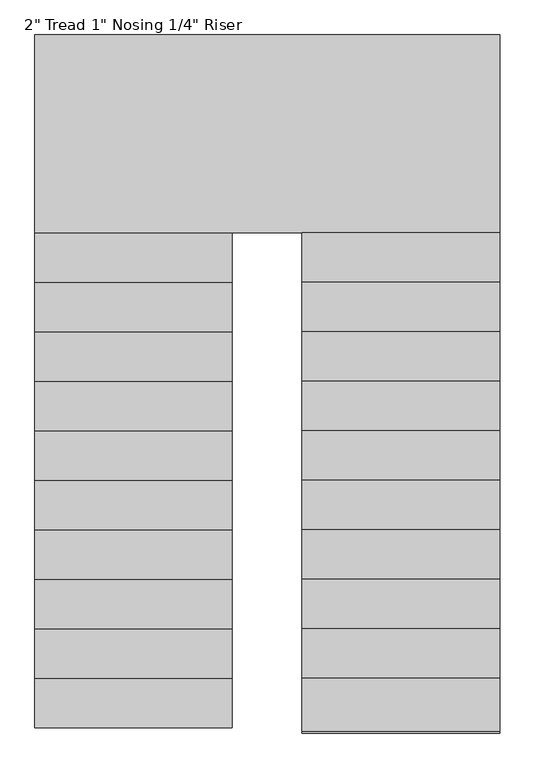
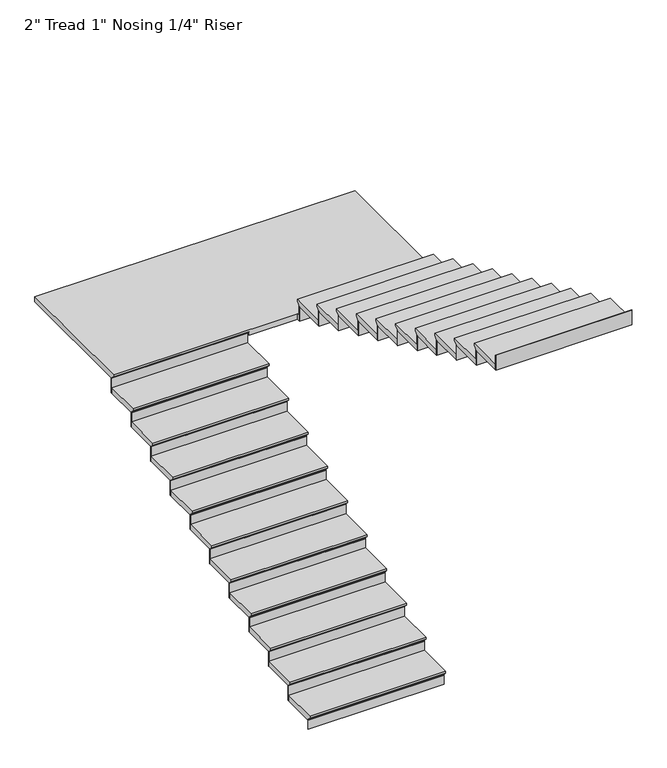
"""IFC4 building model written with IfcOpenShell, lengths in millimetres: stair flight geometry."""

from ifc_helpers import new_model, si_unit, origin, place, context, project, spatial, faceted_brep, source, transform, mapped, element, save


def stair_flight_f8c5991c(model_context):
    return source(origin(), model_context, "Body", "Brep", [
        faceted_brep([(-629.5987998, 3364.6067329, 3319.8954545), (-629.5987998, 3364.6067329, 3338.9454545), (-1845.5417538, 3364.6067329, 3338.9454545), (-1845.5417538, 3364.6067329, 3319.8954545), (-629.5987998, 3390.0067329, 3294.4954545), (-1845.5417538, 3390.0067329, 3294.4954545), (-629.5987998, 3694.8067329, 3338.9454545), (-1845.5417538, 3694.8067329, 3338.9454545), (-1845.5417538, 3390.0067329, 3288.1454545), (-1845.5417538, 3694.8067329, 3288.1454545), (-629.5987998, 3694.8067329, 3288.1454545), (-629.5987998, 3390.0067329, 3288.1454545)], [[[0, 1, 2, 3]], [[4, 0, 3, 5]], [[2, 1, 6, 7]], [[8, 9, 10, 11]], [[2, 7, 9, 8, 5, 3]], [[8, 11, 4, 5]], [[6, 1, 0, 4, 11, 10]], [[7, 6, 10, 9]]]),
        faceted_brep([(-629.5987998, 3390.0067329, 3288.1454545), (-629.5987998, 3390.0067329, 3200.4), (-629.5987998, 3396.3567329, 3200.4), (-629.5987998, 3396.3567329, 3288.1454545), (-1845.5417538, 3390.0067329, 3288.1454545), (-1845.5417538, 3396.3567329, 3288.1454545), (-1845.5417538, 3396.3567329, 3200.4), (-1845.5417538, 3390.0067329, 3200.4)], [[[0, 1, 2, 3]], [[4, 5, 6, 7]], [[1, 0, 4, 7]], [[2, 1, 7, 6]], [[3, 2, 6, 5]], [[0, 3, 5, 4]]]),
        faceted_brep([(-629.5987998, 3694.8067329, 3426.6909091), (-629.5987998, 3694.8067329, 3288.1454545), (-629.5987998, 3701.1567329, 3288.1454545), (-629.5987998, 3701.1567329, 3426.6909091), (-1845.5417538, 3694.8067329, 3426.6909091), (-1845.5417538, 3701.1567329, 3426.6909091), (-1845.5417538, 3701.1567329, 3288.1454545), (-1845.5417538, 3694.8067329, 3288.1454545)], [[[0, 1, 2, 3]], [[4, 5, 6, 7]], [[1, 0, 4, 7]], [[2, 1, 7, 6]], [[3, 2, 6, 5]], [[0, 3, 5, 4]]]),
        faceted_brep([(-1845.5417538, 3669.4067329, 3477.4909091), (-629.5987998, 3669.4067329, 3477.4909091), (-629.5987998, 3999.6067329, 3477.4909091), (-1845.5417538, 3999.6067329, 3477.4909091), (-1845.5417538, 3694.8067329, 3426.6909091), (-1845.5417538, 3999.6067329, 3426.6909091), (-629.5987998, 3999.6067329, 3426.6909091), (-629.5987998, 3694.8067329, 3426.6909091), (-1845.5417538, 3694.8067329, 3433.0409091), (-1845.5417538, 3669.4067329, 3458.4409091), (-629.5987998, 3694.8067329, 3433.0409091), (-629.5987998, 3669.4067329, 3458.4409091)], [[[0, 1, 2, 3]], [[4, 5, 6, 7]], [[0, 3, 5, 4, 8, 9]], [[4, 7, 10, 8]], [[2, 1, 11, 10, 7, 6]], [[3, 2, 6, 5]], [[11, 1, 0, 9]], [[10, 11, 9, 8]]]),
        faceted_brep([(-629.5987998, 3999.6067329, 3565.2363636), (-629.5987998, 3999.6067329, 3426.6909091), (-629.5987998, 4005.9567329, 3426.6909091), (-629.5987998, 4005.9567329, 3565.2363636), (-1845.5417538, 3999.6067329, 3565.2363636), (-1845.5417538, 4005.9567329, 3565.2363636), (-1845.5417538, 4005.9567329, 3426.6909091), (-1845.5417538, 3999.6067329, 3426.6909091)], [[[0, 1, 2, 3]], [[4, 5, 6, 7]], [[1, 0, 4, 7]], [[2, 1, 7, 6]], [[3, 2, 6, 5]], [[0, 3, 5, 4]]]),
        faceted_brep([(-1845.5417538, 3974.2067329, 3616.0363636), (-629.5987998, 3974.2067329, 3616.0363636), (-629.5987998, 4304.4067329, 3616.0363636), (-1845.5417538, 4304.4067329, 3616.0363636), (-1845.5417538, 3999.6067329, 3565.2363636), (-1845.5417538, 4304.4067329, 3565.2363636), (-629.5987998, 4304.4067329, 3565.2363636), (-629.5987998, 3999.6067329, 3565.2363636), (-1845.5417538, 3999.6067329, 3571.5863636), (-1845.5417538, 3974.2067329, 3596.9863636), (-629.5987998, 3999.6067329, 3571.5863636), (-629.5987998, 3974.2067329, 3596.9863636)], [[[0, 1, 2, 3]], [[4, 5, 6, 7]], [[0, 3, 5, 4, 8, 9]], [[4, 7, 10, 8]], [[2, 1, 11, 10, 7, 6]], [[3, 2, 6, 5]], [[11, 1, 0, 9]], [[10, 11, 9, 8]]]),
        faceted_brep([(-629.5987998, 4304.4067329, 3703.7818182), (-629.5987998, 4304.4067329, 3565.2363636), (-629.5987998, 4310.7567329, 3565.2363636), (-629.5987998, 4310.7567329, 3703.7818182), (-1845.5417538, 4304.4067329, 3703.7818182), (-1845.5417538, 4310.7567329, 3703.7818182), (-1845.5417538, 4310.7567329, 3565.2363636), (-1845.5417538, 4304.4067329, 3565.2363636)], [[[0, 1, 2, 3]], [[4, 5, 6, 7]], [[1, 0, 4, 7]], [[2, 1, 7, 6]], [[3, 2, 6, 5]], [[0, 3, 5, 4]]]),
        faceted_brep([(-1845.5417538, 4279.0067329, 3754.5818182), (-629.5987998, 4279.0067329, 3754.5818182), (-629.5987998, 4609.2067329, 3754.5818182), (-1845.5417538, 4609.2067329, 3754.5818182), (-1845.5417538, 4304.4067329, 3703.7818182), (-1845.5417538, 4609.2067329, 3703.7818182), (-629.5987998, 4609.2067329, 3703.7818182), (-629.5987998, 4304.4067329, 3703.7818182), (-1845.5417538, 4304.4067329, 3710.1318182), (-1845.5417538, 4279.0067329, 3735.5318182), (-629.5987998, 4304.4067329, 3710.1318182), (-629.5987998, 4279.0067329, 3735.5318182)], [[[0, 1, 2, 3]], [[4, 5, 6, 7]], [[0, 3, 5, 4, 8, 9]], [[4, 7, 10, 8]], [[2, 1, 11, 10, 7, 6]], [[3, 2, 6, 5]], [[11, 1, 0, 9]], [[10, 11, 9, 8]]]),
        faceted_brep([(-629.5987998, 4609.2067329, 3842.3272727), (-629.5987998, 4609.2067329, 3703.7818182), (-629.5987998, 4615.5567329, 3703.7818182), (-629.5987998, 4615.5567329, 3842.3272727), (-1845.5417538, 4609.2067329, 3842.3272727), (-1845.5417538, 4615.5567329, 3842.3272727), (-1845.5417538, 4615.5567329, 3703.7818182), (-1845.5417538, 4609.2067329, 3703.7818182)], [[[0, 1, 2, 3]], [[4, 5, 6, 7]], [[1, 0, 4, 7]], [[2, 1, 7, 6]], [[3, 2, 6, 5]], [[0, 3, 5, 4]]]),
        faceted_brep([(-1845.5417538, 4583.8067329, 3893.1272727), (-629.5987998, 4583.8067329, 3893.1272727), (-629.5987998, 4914.0067329, 3893.1272727), (-1845.5417538, 4914.0067329, 3893.1272727), (-1845.5417538, 4609.2067329, 3842.3272727), (-1845.5417538, 4914.0067329, 3842.3272727), (-629.5987998, 4914.0067329, 3842.3272727), (-629.5987998, 4609.2067329, 3842.3272727), (-1845.5417538, 4609.2067329, 3848.6772727), (-1845.5417538, 4583.8067329, 3874.0772727), (-629.5987998, 4609.2067329, 3848.6772727), (-629.5987998, 4583.8067329, 3874.0772727)], [[[0, 1, 2, 3]], [[4, 5, 6, 7]], [[0, 3, 5, 4, 8, 9]], [[4, 7, 10, 8]], [[2, 1, 11, 10, 7, 6]], [[3, 2, 6, 5]], [[11, 1, 0, 9]], [[10, 11, 9, 8]]]),
        faceted_brep([(-629.5987998, 4914.0067329, 3980.8727273), (-629.5987998, 4914.0067329, 3842.3272727), (-629.5987998, 4920.3567329, 3842.3272727), (-629.5987998, 4920.3567329, 3980.8727273), (-1845.5417538, 4914.0067329, 3980.8727273), (-1845.5417538, 4920.3567329, 3980.8727273), (-1845.5417538, 4920.3567329, 3842.3272727), (-1845.5417538, 4914.0067329, 3842.3272727)], [[[0, 1, 2, 3]], [[4, 5, 6, 7]], [[1, 0, 4, 7]], [[2, 1, 7, 6]], [[3, 2, 6, 5]], [[0, 3, 5, 4]]]),
        faceted_brep([(-1845.5417538, 4888.6067329, 4031.6727273), (-629.5987998, 4888.6067329, 4031.6727273), (-629.5987998, 5218.8067329, 4031.6727273), (-1845.5417538, 5218.8067329, 4031.6727273), (-1845.5417538, 4914.0067329, 3980.8727273), (-1845.5417538, 5218.8067329, 3980.8727273), (-629.5987998, 5218.8067329, 3980.8727273), (-629.5987998, 4914.0067329, 3980.8727273), (-1845.5417538, 4914.0067329, 3987.2227273), (-1845.5417538, 4888.6067329, 4012.6227273), (-629.5987998, 4914.0067329, 3987.2227273), (-629.5987998, 4888.6067329, 4012.6227273)], [[[0, 1, 2, 3]], [[4, 5, 6, 7]], [[0, 3, 5, 4, 8, 9]], [[4, 7, 10, 8]], [[2, 1, 11, 10, 7, 6]], [[3, 2, 6, 5]], [[11, 1, 0, 9]], [[10, 11, 9, 8]]]),
        faceted_brep([(-629.5987998, 5218.8067329, 4119.4181818), (-629.5987998, 5218.8067329, 3980.8727273), (-629.5987998, 5225.1567329, 3980.8727273), (-629.5987998, 5225.1567329, 4119.4181818), (-1845.5417538, 5218.8067329, 4119.4181818), (-1845.5417538, 5225.1567329, 4119.4181818), (-1845.5417538, 5225.1567329, 3980.8727273), (-1845.5417538, 5218.8067329, 3980.8727273)], [[[0, 1, 2, 3]], [[4, 5, 6, 7]], [[1, 0, 4, 7]], [[2, 1, 7, 6]], [[3, 2, 6, 5]], [[0, 3, 5, 4]]]),
        faceted_brep([(-1845.5417538, 5193.4067329, 4170.2181818), (-629.5987998, 5193.4067329, 4170.2181818), (-629.5987998, 5523.6067329, 4170.2181818), (-1845.5417538, 5523.6067329, 4170.2181818), (-1845.5417538, 5218.8067329, 4119.4181818), (-1845.5417538, 5523.6067329, 4119.4181818), (-629.5987998, 5523.6067329, 4119.4181818), (-629.5987998, 5218.8067329, 4119.4181818), (-1845.5417538, 5218.8067329, 4125.7681818), (-1845.5417538, 5193.4067329, 4151.1681818), (-629.5987998, 5218.8067329, 4125.7681818), (-629.5987998, 5193.4067329, 4151.1681818)], [[[0, 1, 2, 3]], [[4, 5, 6, 7]], [[0, 3, 5, 4, 8, 9]], [[4, 7, 10, 8]], [[2, 1, 11, 10, 7, 6]], [[3, 2, 6, 5]], [[11, 1, 0, 9]], [[10, 11, 9, 8]]]),
        faceted_brep([(-629.5987998, 5523.6067329, 4257.9636364), (-629.5987998, 5523.6067329, 4119.4181818), (-629.5987998, 5529.9567329, 4119.4181818), (-629.5987998, 5529.9567329, 4257.9636364), (-1845.5417538, 5523.6067329, 4257.9636364), (-1845.5417538, 5529.9567329, 4257.9636364), (-1845.5417538, 5529.9567329, 4119.4181818), (-1845.5417538, 5523.6067329, 4119.4181818)], [[[0, 1, 2, 3]], [[4, 5, 6, 7]], [[1, 0, 4, 7]], [[2, 1, 7, 6]], [[3, 2, 6, 5]], [[0, 3, 5, 4]]]),
        faceted_brep([(-1845.5417538, 5498.2067329, 4308.7636364), (-629.5987998, 5498.2067329, 4308.7636364), (-629.5987998, 5828.4067329, 4308.7636364), (-1845.5417538, 5828.4067329, 4308.7636364), (-1845.5417538, 5523.6067329, 4257.9636364), (-1845.5417538, 5828.4067329, 4257.9636364), (-629.5987998, 5828.4067329, 4257.9636364), (-629.5987998, 5523.6067329, 4257.9636364), (-1845.5417538, 5523.6067329, 4264.3136364), (-1845.5417538, 5498.2067329, 4289.7136364), (-629.5987998, 5523.6067329, 4264.3136364), (-629.5987998, 5498.2067329, 4289.7136364)], [[[0, 1, 2, 3]], [[4, 5, 6, 7]], [[0, 3, 5, 4, 8, 9]], [[4, 7, 10, 8]], [[2, 1, 11, 10, 7, 6]], [[3, 2, 6, 5]], [[11, 1, 0, 9]], [[10, 11, 9, 8]]]),
        faceted_brep([(-629.5987998, 5828.4067329, 4396.5090909), (-629.5987998, 5828.4067329, 4257.9636364), (-629.5987998, 5834.7567329, 4257.9636364), (-629.5987998, 5834.7567329, 4396.5090909), (-1845.5417538, 5828.4067329, 4396.5090909), (-1845.5417538, 5834.7567329, 4396.5090909), (-1845.5417538, 5834.7567329, 4257.9636364), (-1845.5417538, 5828.4067329, 4257.9636364)], [[[0, 1, 2, 3]], [[4, 5, 6, 7]], [[1, 0, 4, 7]], [[2, 1, 7, 6]], [[3, 2, 6, 5]], [[0, 3, 5, 4]]]),
        faceted_brep([(-1845.5417538, 5803.0067329, 4447.3090909), (-629.5987998, 5803.0067329, 4447.3090909), (-629.5987998, 6133.2067329, 4447.3090909), (-1845.5417538, 6133.2067329, 4447.3090909), (-1845.5417538, 5828.4067329, 4396.5090909), (-1845.5417538, 6133.2067329, 4396.5090909), (-629.5987998, 6133.2067329, 4396.5090909), (-629.5987998, 5828.4067329, 4396.5090909), (-1845.5417538, 5828.4067329, 4402.8590909), (-1845.5417538, 5803.0067329, 4428.2590909), (-629.5987998, 5828.4067329, 4402.8590909), (-629.5987998, 5803.0067329, 4428.2590909)], [[[0, 1, 2, 3]], [[4, 5, 6, 7]], [[0, 3, 5, 4, 8, 9]], [[4, 7, 10, 8]], [[2, 1, 11, 10, 7, 6]], [[3, 2, 6, 5]], [[11, 1, 0, 9]], [[10, 11, 9, 8]]]),
        faceted_brep([(-629.5987998, 6133.2067329, 4535.0545455), (-629.5987998, 6133.2067329, 4396.5090909), (-629.5987998, 6139.5567329, 4396.5090909), (-629.5987998, 6139.5567329, 4535.0545455), (-1845.5417538, 6133.2067329, 4535.0545455), (-1845.5417538, 6139.5567329, 4535.0545455), (-1845.5417538, 6139.5567329, 4396.5090909), (-1845.5417538, 6133.2067329, 4396.5090909)], [[[0, 1, 2, 3]], [[4, 5, 6, 7]], [[1, 0, 4, 7]], [[2, 1, 7, 6]], [[3, 2, 6, 5]], [[0, 3, 5, 4]]]),
        faceted_brep([(-1845.5417538, 6107.8067329, 4585.8545455), (-629.5987998, 6107.8067329, 4585.8545455), (-629.5987998, 6438.0067329, 4585.8545455), (-1845.5417538, 6438.0067329, 4585.8545455), (-1845.5417538, 6133.2067329, 4535.0545455), (-1845.5417538, 6438.0067329, 4535.0545455), (-629.5987998, 6438.0067329, 4535.0545455), (-629.5987998, 6133.2067329, 4535.0545455), (-1845.5417538, 6133.2067329, 4541.4045455), (-1845.5417538, 6107.8067329, 4566.8045455), (-629.5987998, 6133.2067329, 4541.4045455), (-629.5987998, 6107.8067329, 4566.8045455)], [[[0, 1, 2, 3]], [[4, 5, 6, 7]], [[0, 3, 5, 4, 8, 9]], [[4, 7, 10, 8]], [[2, 1, 11, 10, 7, 6]], [[3, 2, 6, 5]], [[11, 1, 0, 9]], [[10, 11, 9, 8]]]),
        faceted_brep([(-629.5987998, 6438.0067329, 4673.6), (-629.5987998, 6438.0067329, 4535.0545455), (-629.5987998, 6444.3567329, 4535.0545455), (-629.5987998, 6444.3567329, 4673.6), (-1845.5417538, 6438.0067329, 4673.6), (-1845.5417538, 6444.3567329, 4673.6), (-1845.5417538, 6444.3567329, 4535.0545455), (-1845.5417538, 6438.0067329, 4535.0545455)], [[[0, 1, 2, 3]], [[4, 5, 6, 7]], [[1, 0, 4, 7]], [[2, 1, 7, 6]], [[3, 2, 6, 5]], [[0, 3, 5, 4]]]),
        faceted_brep([(1021.4012085, 6387.2067329, 4724.4), (1021.4012085, 7631.8067329, 4724.4), (-1845.5417538, 7631.8067329, 4724.4), (-1845.5417538, 6412.6067329, 4724.4), (-197.7987915, 6412.6067329, 4724.4), (-197.7987915, 6387.2067329, 4724.4), (1021.4012085, 7631.8067329, 4673.6), (1021.4012085, 6387.2067329, 4673.6), (-197.7987915, 6387.2067329, 4673.6), (-197.7987915, 6412.6067329, 4673.6), (-629.5987998, 6412.6067329, 4673.6), (-629.5987998, 6438.0067329, 4673.6), (-1845.5417538, 6438.0067329, 4673.6), (-1845.5417538, 7631.8067329, 4673.6), (-629.5987998, 6438.0067329, 4679.95), (-1845.5417538, 6438.0067329, 4679.95), (-1845.5417538, 6412.6067329, 4705.35), (-629.5987998, 6412.6067329, 4705.35)], [[[0, 1, 2, 3, 4, 5]], [[6, 7, 8, 9, 10, 11, 12, 13]], [[1, 0, 7, 6]], [[2, 1, 6, 13]], [[12, 11, 14, 15]], [[4, 3, 16, 17, 10, 9]], [[5, 4, 9, 8]], [[0, 5, 8, 7]], [[16, 15, 14, 17]], [[3, 2, 13, 12, 15, 16]], [[11, 10, 17, 14]]]),
        faceted_brep([(-197.7987915, 6387.2067329, 4812.1454545), (-197.7987915, 6387.2067329, 4673.6), (-197.7987915, 6380.8567329, 4673.6), (-197.7987915, 6380.8567329, 4812.1454545), (1021.4012085, 6387.2067329, 4812.1454545), (1021.4012085, 6380.8567329, 4812.1454545), (1021.4012085, 6380.8567329, 4673.6), (1021.4012085, 6387.2067329, 4673.6)], [[[0, 1, 2, 3]], [[4, 5, 6, 7]], [[1, 0, 4, 7]], [[2, 1, 7, 6]], [[3, 2, 6, 5]], [[0, 3, 5, 4]]]),
        faceted_brep([(1021.4012085, 6412.6067329, 4862.9454545), (-197.7987915, 6412.6067329, 4862.9454545), (-197.7987915, 6082.4067329, 4862.9454545), (1021.4012085, 6082.4067329, 4862.9454545), (1021.4012085, 6387.2067329, 4812.1454545), (1021.4012085, 6082.4067329, 4812.1454545), (-197.7987915, 6082.4067329, 4812.1454545), (-197.7987915, 6387.2067329, 4812.1454545), (1021.4012085, 6387.2067329, 4818.4954545), (1021.4012085, 6412.6067329, 4843.8954545), (-197.7987915, 6387.2067329, 4818.4954545), (-197.7987915, 6412.6067329, 4843.8954545)], [[[0, 1, 2, 3]], [[4, 5, 6, 7]], [[0, 3, 5, 4, 8, 9]], [[4, 7, 10, 8]], [[2, 1, 11, 10, 7, 6]], [[3, 2, 6, 5]], [[11, 1, 0, 9]], [[10, 11, 9, 8]]]),
        faceted_brep([(-197.7987915, 6082.4067329, 4950.6909091), (-197.7987915, 6082.4067329, 4812.1454545), (-197.7987915, 6076.0567329, 4812.1454545), (-197.7987915, 6076.0567329, 4950.6909091), (1021.4012085, 6082.4067329, 4950.6909091), (1021.4012085, 6076.0567329, 4950.6909091), (1021.4012085, 6076.0567329, 4812.1454545), (1021.4012085, 6082.4067329, 4812.1454545)], [[[0, 1, 2, 3]], [[4, 5, 6, 7]], [[1, 0, 4, 7]], [[2, 1, 7, 6]], [[3, 2, 6, 5]], [[0, 3, 5, 4]]]),
        faceted_brep([(1021.4012085, 6107.8067329, 5001.4909091), (-197.7987915, 6107.8067329, 5001.4909091), (-197.7987915, 5777.6067329, 5001.4909091), (1021.4012085, 5777.6067329, 5001.4909091), (1021.4012085, 6082.4067329, 4950.6909091), (1021.4012085, 5777.6067329, 4950.6909091), (-197.7987915, 5777.6067329, 4950.6909091), (-197.7987915, 6082.4067329, 4950.6909091), (1021.4012085, 6082.4067329, 4957.0409091), (1021.4012085, 6107.8067329, 4982.4409091), (-197.7987915, 6082.4067329, 4957.0409091), (-197.7987915, 6107.8067329, 4982.4409091)], [[[0, 1, 2, 3]], [[4, 5, 6, 7]], [[0, 3, 5, 4, 8, 9]], [[4, 7, 10, 8]], [[2, 1, 11, 10, 7, 6]], [[3, 2, 6, 5]], [[11, 1, 0, 9]], [[10, 11, 9, 8]]]),
        faceted_brep([(-197.7987915, 5777.6067329, 5089.2363636), (-197.7987915, 5777.6067329, 4950.6909091), (-197.7987915, 5771.2567329, 4950.6909091), (-197.7987915, 5771.2567329, 5089.2363636), (1021.4012085, 5777.6067329, 5089.2363636), (1021.4012085, 5771.2567329, 5089.2363636), (1021.4012085, 5771.2567329, 4950.6909091), (1021.4012085, 5777.6067329, 4950.6909091)], [[[0, 1, 2, 3]], [[4, 5, 6, 7]], [[1, 0, 4, 7]], [[2, 1, 7, 6]], [[3, 2, 6, 5]], [[0, 3, 5, 4]]]),
        faceted_brep([(1021.4012085, 5803.0067329, 5140.0363636), (-197.7987915, 5803.0067329, 5140.0363636), (-197.7987915, 5472.8067329, 5140.0363636), (1021.4012085, 5472.8067329, 5140.0363636), (1021.4012085, 5777.6067329, 5089.2363636), (1021.4012085, 5472.8067329, 5089.2363636), (-197.7987915, 5472.8067329, 5089.2363636), (-197.7987915, 5777.6067329, 5089.2363636), (1021.4012085, 5777.6067329, 5095.5863636), (1021.4012085, 5803.0067329, 5120.9863636), (-197.7987915, 5777.6067329, 5095.5863636), (-197.7987915, 5803.0067329, 5120.9863636)], [[[0, 1, 2, 3]], [[4, 5, 6, 7]], [[0, 3, 5, 4, 8, 9]], [[4, 7, 10, 8]], [[2, 1, 11, 10, 7, 6]], [[3, 2, 6, 5]], [[11, 1, 0, 9]], [[10, 11, 9, 8]]]),
        faceted_brep([(-197.7987915, 5472.8067329, 5227.7818182), (-197.7987915, 5472.8067329, 5089.2363636), (-197.7987915, 5466.4567329, 5089.2363636), (-197.7987915, 5466.4567329, 5227.7818182), (1021.4012085, 5472.8067329, 5227.7818182), (1021.4012085, 5466.4567329, 5227.7818182), (1021.4012085, 5466.4567329, 5089.2363636), (1021.4012085, 5472.8067329, 5089.2363636)], [[[0, 1, 2, 3]], [[4, 5, 6, 7]], [[1, 0, 4, 7]], [[2, 1, 7, 6]], [[3, 2, 6, 5]], [[0, 3, 5, 4]]]),
        faceted_brep([(1021.4012085, 5498.2067329, 5278.5818182), (-197.7987915, 5498.2067329, 5278.5818182), (-197.7987915, 5168.0067329, 5278.5818182), (1021.4012085, 5168.0067329, 5278.5818182), (1021.4012085, 5472.8067329, 5227.7818182), (1021.4012085, 5168.0067329, 5227.7818182), (-197.7987915, 5168.0067329, 5227.7818182), (-197.7987915, 5472.8067329, 5227.7818182), (1021.4012085, 5472.8067329, 5234.1318182), (1021.4012085, 5498.2067329, 5259.5318182), (-197.7987915, 5472.8067329, 5234.1318182), (-197.7987915, 5498.2067329, 5259.5318182)], [[[0, 1, 2, 3]], [[4, 5, 6, 7]], [[0, 3, 5, 4, 8, 9]], [[4, 7, 10, 8]], [[2, 1, 11, 10, 7, 6]], [[3, 2, 6, 5]], [[11, 1, 0, 9]], [[10, 11, 9, 8]]]),
        faceted_brep([(-197.7987915, 5168.0067329, 5366.3272727), (-197.7987915, 5168.0067329, 5227.7818182), (-197.7987915, 5161.6567329, 5227.7818182), (-197.7987915, 5161.6567329, 5366.3272727), (1021.4012085, 5168.0067329, 5366.3272727), (1021.4012085, 5161.6567329, 5366.3272727), (1021.4012085, 5161.6567329, 5227.7818182), (1021.4012085, 5168.0067329, 5227.7818182)], [[[0, 1, 2, 3]], [[4, 5, 6, 7]], [[1, 0, 4, 7]], [[2, 1, 7, 6]], [[3, 2, 6, 5]], [[0, 3, 5, 4]]]),
        faceted_brep([(1021.4012085, 5193.4067329, 5417.1272727), (-197.7987915, 5193.4067329, 5417.1272727), (-197.7987915, 4863.2067329, 5417.1272727), (1021.4012085, 4863.2067329, 5417.1272727), (1021.4012085, 5168.0067329, 5366.3272727), (1021.4012085, 4863.2067329, 5366.3272727), (-197.7987915, 4863.2067329, 5366.3272727), (-197.7987915, 5168.0067329, 5366.3272727), (1021.4012085, 5168.0067329, 5372.6772727), (1021.4012085, 5193.4067329, 5398.0772727), (-197.7987915, 5168.0067329, 5372.6772727), (-197.7987915, 5193.4067329, 5398.0772727)], [[[0, 1, 2, 3]], [[4, 5, 6, 7]], [[0, 3, 5, 4, 8, 9]], [[4, 7, 10, 8]], [[2, 1, 11, 10, 7, 6]], [[3, 2, 6, 5]], [[11, 1, 0, 9]], [[10, 11, 9, 8]]]),
        faceted_brep([(-197.7987915, 4863.2067329, 5504.8727273), (-197.7987915, 4863.2067329, 5366.3272727), (-197.7987915, 4856.8567329, 5366.3272727), (-197.7987915, 4856.8567329, 5504.8727273), (1021.4012085, 4863.2067329, 5504.8727273), (1021.4012085, 4856.8567329, 5504.8727273), (1021.4012085, 4856.8567329, 5366.3272727), (1021.4012085, 4863.2067329, 5366.3272727)], [[[0, 1, 2, 3]], [[4, 5, 6, 7]], [[1, 0, 4, 7]], [[2, 1, 7, 6]], [[3, 2, 6, 5]], [[0, 3, 5, 4]]]),
        faceted_brep([(1021.4012085, 4888.6067329, 5555.6727273), (-197.7987915, 4888.6067329, 5555.6727273), (-197.7987915, 4558.4067329, 5555.6727273), (1021.4012085, 4558.4067329, 5555.6727273), (1021.4012085, 4863.2067329, 5504.8727273), (1021.4012085, 4558.4067329, 5504.8727273), (-197.7987915, 4558.4067329, 5504.8727273), (-197.7987915, 4863.2067329, 5504.8727273), (1021.4012085, 4863.2067329, 5511.2227273), (1021.4012085, 4888.6067329, 5536.6227273), (-197.7987915, 4863.2067329, 5511.2227273), (-197.7987915, 4888.6067329, 5536.6227273)], [[[0, 1, 2, 3]], [[4, 5, 6, 7]], [[0, 3, 5, 4, 8, 9]], [[4, 7, 10, 8]], [[2, 1, 11, 10, 7, 6]], [[3, 2, 6, 5]], [[11, 1, 0, 9]], [[10, 11, 9, 8]]]),
        faceted_brep([(-197.7987915, 4558.4067329, 5643.4181818), (-197.7987915, 4558.4067329, 5504.8727273), (-197.7987915, 4552.0567329, 5504.8727273), (-197.7987915, 4552.0567329, 5643.4181818), (1021.4012085, 4558.4067329, 5643.4181818), (1021.4012085, 4552.0567329, 5643.4181818), (1021.4012085, 4552.0567329, 5504.8727273), (1021.4012085, 4558.4067329, 5504.8727273)], [[[0, 1, 2, 3]], [[4, 5, 6, 7]], [[1, 0, 4, 7]], [[2, 1, 7, 6]], [[3, 2, 6, 5]], [[0, 3, 5, 4]]]),
        faceted_brep([(1021.4012085, 4583.8067329, 5694.2181818), (-197.7987915, 4583.8067329, 5694.2181818), (-197.7987915, 4253.6067329, 5694.2181818), (1021.4012085, 4253.6067329, 5694.2181818), (1021.4012085, 4558.4067329, 5643.4181818), (1021.4012085, 4253.6067329, 5643.4181818), (-197.7987915, 4253.6067329, 5643.4181818), (-197.7987915, 4558.4067329, 5643.4181818), (1021.4012085, 4558.4067329, 5649.7681818), (1021.4012085, 4583.8067329, 5675.1681818), (-197.7987915, 4558.4067329, 5649.7681818), (-197.7987915, 4583.8067329, 5675.1681818)], [[[0, 1, 2, 3]], [[4, 5, 6, 7]], [[0, 3, 5, 4, 8, 9]], [[4, 7, 10, 8]], [[2, 1, 11, 10, 7, 6]], [[3, 2, 6, 5]], [[11, 1, 0, 9]], [[10, 11, 9, 8]]]),
        faceted_brep([(-197.7987915, 4253.6067329, 5781.9636364), (-197.7987915, 4253.6067329, 5643.4181818), (-197.7987915, 4247.2567329, 5643.4181818), (-197.7987915, 4247.2567329, 5781.9636364), (1021.4012085, 4253.6067329, 5781.9636364), (1021.4012085, 4247.2567329, 5781.9636364), (1021.4012085, 4247.2567329, 5643.4181818), (1021.4012085, 4253.6067329, 5643.4181818)], [[[0, 1, 2, 3]], [[4, 5, 6, 7]], [[1, 0, 4, 7]], [[2, 1, 7, 6]], [[3, 2, 6, 5]], [[0, 3, 5, 4]]]),
        faceted_brep([(1021.4012085, 4279.0067329, 5832.7636364), (-197.7987915, 4279.0067329, 5832.7636364), (-197.7987915, 3948.8067329, 5832.7636364), (1021.4012085, 3948.8067329, 5832.7636364), (1021.4012085, 4253.6067329, 5781.9636364), (1021.4012085, 3948.8067329, 5781.9636364), (-197.7987915, 3948.8067329, 5781.9636364), (-197.7987915, 4253.6067329, 5781.9636364), (1021.4012085, 4253.6067329, 5788.3136364), (1021.4012085, 4279.0067329, 5813.7136364), (-197.7987915, 4253.6067329, 5788.3136364), (-197.7987915, 4279.0067329, 5813.7136364)], [[[0, 1, 2, 3]], [[4, 5, 6, 7]], [[0, 3, 5, 4, 8, 9]], [[4, 7, 10, 8]], [[2, 1, 11, 10, 7, 6]], [[3, 2, 6, 5]], [[11, 1, 0, 9]], [[10, 11, 9, 8]]]),
        faceted_brep([(-197.7987915, 3948.8067329, 5920.5090909), (-197.7987915, 3948.8067329, 5781.9636364), (-197.7987915, 3942.4567329, 5781.9636364), (-197.7987915, 3942.4567329, 5920.5090909), (1021.4012085, 3948.8067329, 5920.5090909), (1021.4012085, 3942.4567329, 5920.5090909), (1021.4012085, 3942.4567329, 5781.9636364), (1021.4012085, 3948.8067329, 5781.9636364)], [[[0, 1, 2, 3]], [[4, 5, 6, 7]], [[1, 0, 4, 7]], [[2, 1, 7, 6]], [[3, 2, 6, 5]], [[0, 3, 5, 4]]]),
        faceted_brep([(1021.4012085, 3974.2067329, 5971.3090909), (-197.7987915, 3974.2067329, 5971.3090909), (-197.7987915, 3644.0067329, 5971.3090909), (1021.4012085, 3644.0067329, 5971.3090909), (1021.4012085, 3948.8067329, 5920.5090909), (1021.4012085, 3644.0067329, 5920.5090909), (-197.7987915, 3644.0067329, 5920.5090909), (-197.7987915, 3948.8067329, 5920.5090909), (1021.4012085, 3948.8067329, 5926.8590909), (1021.4012085, 3974.2067329, 5952.2590909), (-197.7987915, 3948.8067329, 5926.8590909), (-197.7987915, 3974.2067329, 5952.2590909)], [[[0, 1, 2, 3]], [[4, 5, 6, 7]], [[0, 3, 5, 4, 8, 9]], [[4, 7, 10, 8]], [[2, 1, 11, 10, 7, 6]], [[3, 2, 6, 5]], [[11, 1, 0, 9]], [[10, 11, 9, 8]]]),
        faceted_brep([(-197.7987915, 3644.0067329, 6059.0545455), (-197.7987915, 3644.0067329, 5920.5090909), (-197.7987915, 3637.6567329, 5920.5090909), (-197.7987915, 3637.6567329, 6059.0545455), (1021.4012085, 3644.0067329, 6059.0545455), (1021.4012085, 3637.6567329, 6059.0545455), (1021.4012085, 3637.6567329, 5920.5090909), (1021.4012085, 3644.0067329, 5920.5090909)], [[[0, 1, 2, 3]], [[4, 5, 6, 7]], [[1, 0, 4, 7]], [[2, 1, 7, 6]], [[3, 2, 6, 5]], [[0, 3, 5, 4]]]),
        faceted_brep([(-197.7987915, 3339.2067329, 6197.6), (-197.7987915, 3339.2067329, 6059.0545455), (-197.7987915, 3332.8567329, 6059.0545455), (-197.7987915, 3332.8567329, 6197.6), (1021.4012085, 3339.2067329, 6197.6), (1021.4012085, 3332.8567329, 6197.6), (1021.4012085, 3332.8567329, 6059.0545455), (1021.4012085, 3339.2067329, 6059.0545455)], [[[0, 1, 2, 3]], [[4, 5, 6, 7]], [[1, 0, 4, 7]], [[2, 1, 7, 6]], [[3, 2, 6, 5]], [[0, 3, 5, 4]]]),
        faceted_brep([(1021.4012085, 3669.4067329, 6109.8545455), (-197.7987915, 3669.4067329, 6109.8545455), (-197.7987915, 3339.2067329, 6109.8545455), (1021.4012085, 3339.2067329, 6109.8545455), (1021.4012085, 3644.0067329, 6059.0545455), (1021.4012085, 3339.2067329, 6059.0545455), (-197.7987915, 3339.2067329, 6059.0545455), (-197.7987915, 3644.0067329, 6059.0545455), (1021.4012085, 3644.0067329, 6065.4045455), (1021.4012085, 3669.4067329, 6090.8045455), (-197.7987915, 3644.0067329, 6065.4045455), (-197.7987915, 3669.4067329, 6090.8045455)], [[[0, 1, 2, 3]], [[4, 5, 6, 7]], [[0, 3, 5, 4, 8, 9]], [[4, 7, 10, 8]], [[2, 1, 11, 10, 7, 6]], [[3, 2, 6, 5]], [[11, 1, 0, 9]], [[10, 11, 9, 8]]]),
    ])


if __name__ == "__main__":
    model = new_model("IFC4")
    model_context = context("Model", 3, world=origin())
    ifc_project = project(units=[si_unit("LENGTHUNIT", "METRE", prefix="MILLI")], contexts=[model_context])
    site = spatial("IfcSite", under=ifc_project)
    building = spatial("IfcBuilding", under=site)
    placement = place(None, origin())
    stair_flight_shape = stair_flight_f8c5991c(model_context)
    element("IfcStairFlight", 1, ObjectType="2\" Tread 1\" Nosing 1/4\" Riser", at=placement, inside=building, context=model_context, shape_type="MappedRepresentation", body=[
        mapped(stair_flight_shape, transform((0.0, 0.0, 0.0), x_axis=(1.0, 0.0, 0.0), y_axis=(0.0, 1.0, 0.0), z_axis=(0.0, 0.0, 1.0))),
    ])
    save(model, "model.ifc")
